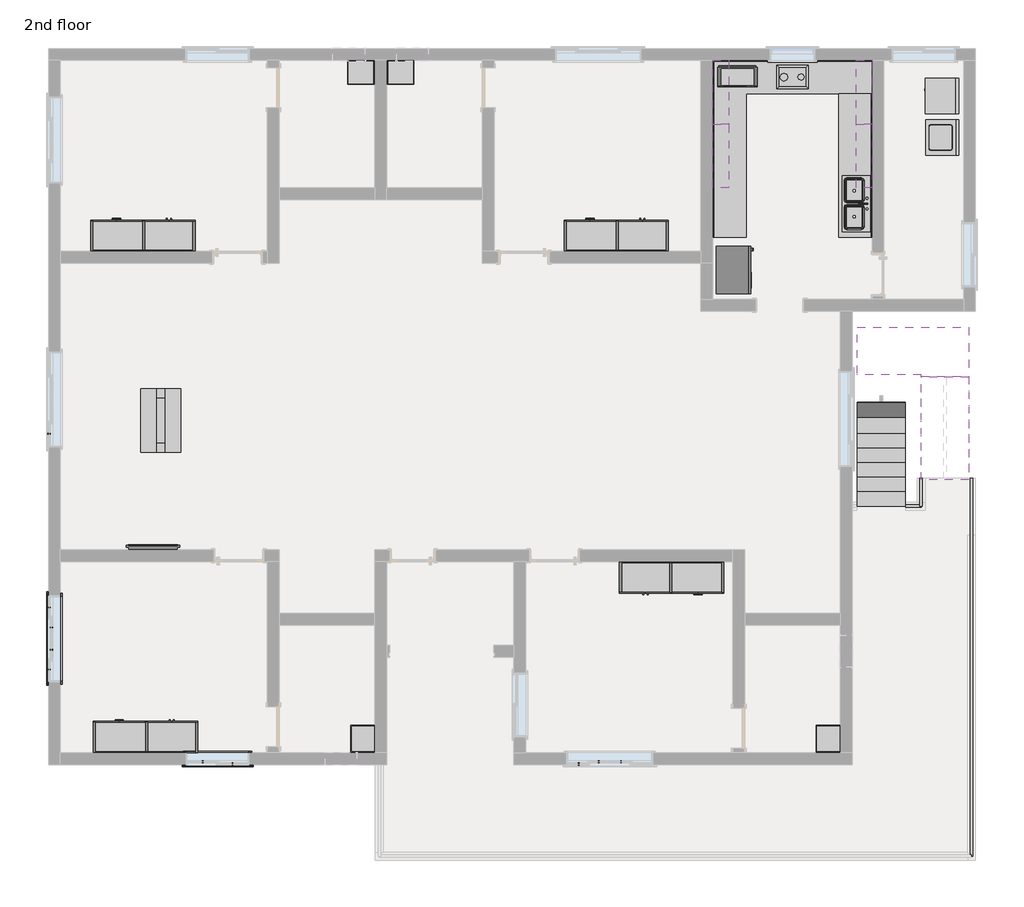
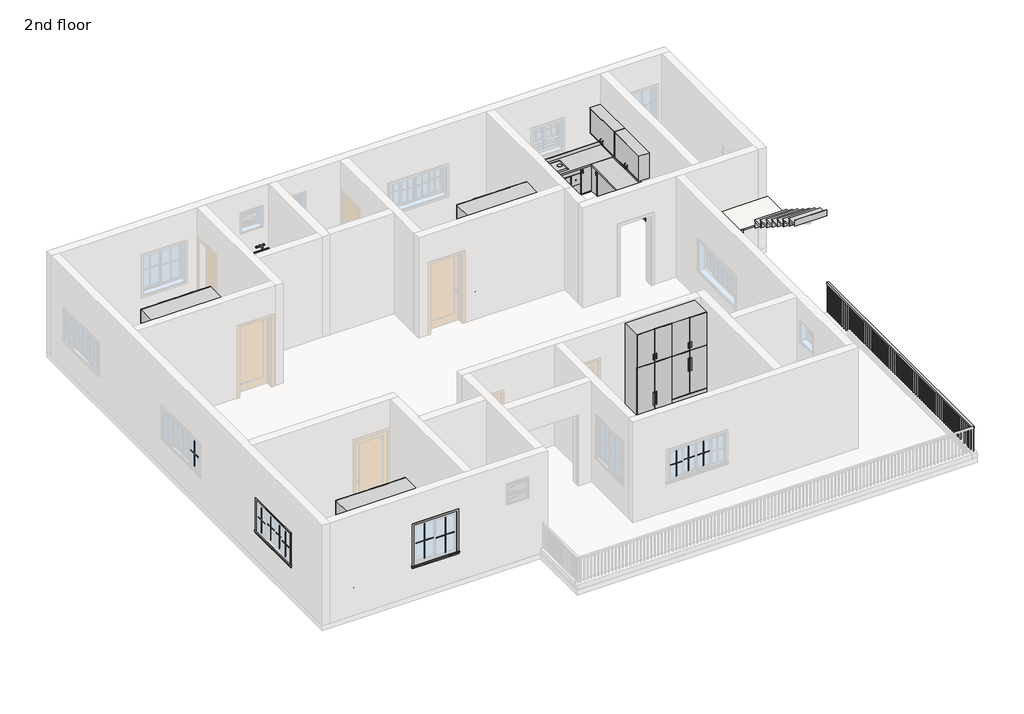
# One storey, part 3 of 4: 19 furniture elements, 18 proxies, 5 flow terminals, 3 railings, 2 stair flights, 1 slab.
# Revit data of these elements (continued)
# Elements 12, 13 (IfcBuildingElementProxy, "Muntin Pattern_2x2 : Muntin Pattern_2x2")
#   Width = 1' - 8 5/8"
#   Height = 3' - 6 1/4"
#   Interior Material = Wood - Stained
#   Exterior Material = Clad - White
#   Phase Created = New Construction
#   Materials on its faces: "Clad - White", "Wood - Stained"
# Element 14 (IfcBuildingElementProxy, "Trim-Window-Exterior-Flat : with Sill")
#   Opening Width = 5' - 5"
#   Opening Height = 3' - 0"
#   Trim Material = Clad - White
#   Phase Created = New Construction
#   Materials on its faces: "Clad - White"
# Element 15 (IfcBuildingElementProxy, "Trim-Window-Exterior-Flat : with Sill")
#   Opening Width = 4' - 0"
#   Opening Height = 4' - 0"
#   Trim Material = Clad - White
#   Phase Created = New Construction
#   Materials on its faces: "Clad - White"
# Element 16 (IfcBuildingElementProxy, "Trim-Window-Interior-Flat : Picture Frame")
#   Opening Width = 5' - 5"
#   Opening Height = 3' - 0"
#   Trim Material = Wood - Stained
#   Phase Created = New Construction
#   Materials on its faces: "Wood - Stained"
# Element 17 (IfcBuildingElementProxy, "Trim-Window-Interior-Flat : Picture Frame")
#   Opening Width = 4' - 0"
#   Opening Height = 4' - 0"
#   Trim Material = Wood - Stained
#   Phase Created = New Construction
#   Materials on its faces: "Wood - Stained"
# Element 18 (IfcBuildingElementProxy, "Washer : 27\" x 25\" x 35\"")
#   Phase Created = New Construction
#   Materials on its faces: "Metal - Paint Finish - Ivory,Matte"
# Element 19 (IfcFlowTerminal, "Sink - Work : 20\"x18\"")
#   Mark = "32"
#   Flow Pressure = 8.00 psi
#   Phase Created = New Construction
# Element 20 (IfcFlowTerminal, "Sink - Work : 20\"x18\"")
#   Mark = "33"
#   Flow Pressure = 8.00 psi
#   Phase Created = New Construction
# Element 21 (IfcFlowTerminal, "Sink - Work : 20\"x18\"")
#   Mark = "34"
#   Flow Pressure = 8.00 psi
#   Phase Created = New Construction
# Element 22 (IfcFlowTerminal, "Sink - Work : 20\"x18\"")
#   Mark = "35"
#   Flow Pressure = 8.00 psi
#   Phase Created = New Construction
# Element 23 (IfcFlowTerminal, "Sink Kitchen-Double : 42\" x 21\"")
#   Mark = "27"
#   Phase Created = New Construction
#   Materials on its faces: "Steel, Polished"
# Element 24 (IfcFurniture)
#   Phase Created = New Construction
#   Materials on its faces: "Default", "Default 3", "Default 2"
# Elements 25, 26, 27, 28 (IfcFurniture, "1Wardrobe_6271 : 1Wardrobe_6271")
#   Phase Created = New Construction
#   Materials on its faces: "Phase - Demo", "Default Wall", "Phase - Exist", "Default"
# Elements 29, 30, 31, 32 (IfcFurniture, "48\" 2")
#   Phase Created = New Construction
#   Materials on its faces: "Cabinets", "Cabinets - Handles"
# Elements 33, 34 (IfcFurniture, "Base Cabinet-Corner Unit-Square : 36\"")
#   Phase Created = New Construction
#   Materials on its faces: "Cabinets", "Cabinets - Handles"
# Element 35 (IfcFurniture, "Counter Top w Sink : 24\" Depth")
#   Sink Opening Width = 3' - 3"
#   Sink Opening Depth = 1' - 3"
#   Sink Location To Wall = 0' - 6"
#   Sink Location = 6' - 11"
#   Length = 9' - 0.36336"
#   Phase Created = New Construction
#   Materials on its faces: "Counter Top"
# Element 36 (IfcFurniture, "Counter Top-L Shaped : 24\" Depth")
#   Length - Leg 2 = 11' - 1.36336"
#   Length - Leg 1 = 10' - 0"
#   Phase Created = New Construction
#   Materials on its faces: "Counter Top"
# Element 37 (IfcFurniture, "Television-Plasma : 42\"")
#   Phase Created = New Construction
#   Materials on its faces: "Plastic - Gray", "Glass"
# Elements 38, 39, 40, 41 (IfcFurniture, "Upper Cabinet-Pass-Thru : 48\" x 30\" x 12\"")
#   Phase Created = New Construction
#   Materials on its faces: "Cabinet"
# Element 42 (IfcFurniture, "White_Modern_Coffee_Table_17067 : White_Modern_Coffee_Table_17067")
#   Phase Created = New Construction
#   Materials on its faces: "White Modern Coffee Table - Plastic", "White Modern Coffee Table - Wood"
# Elements 43, 44, 45 (IfcRailing, "Handrail - Rectangular")
#   Phase Created = New Construction
# Element 46 (IfcSlab, "Non-Monolithic Landing")
#   Phase Created = New Construction
# Elements 47, 48 (IfcStairFlight, "2\" Tread 1\" Nosing 1/4\" Riser")
#   Phase Created = New Construction
# Materials
#   "Metal - Chrome": colour RGB 17 17 17, transparency 0
#   "Metal - Steel, Polished": colour RGB 57 57 57, transparency 0
#   "Metal - Paint Finish - Ivory,Glossy": colour RGB 247 247 239, transparency 0
#   "Laminate - Ivory,Matte": colour RGB 247 247 239, transparency 0
#   "Metal - Paint Finish - Ivory,Matte": colour RGB 247 247 239, transparency 0
#   "Steel, Polished": class "Metal", colour RGB 192 192 192, transparency 0, Description = "Polished steel", Cost = 0
#   "Cabinets - Handles": class "Metal", colour RGB 57 57 57, transparency 0
#   "Cabinets": colour RGB 249 249 249, transparency 0
#   "Plastic - Gray": colour RGB 134 134 134, transparency 0
#   "White Modern Coffee Table - Wood": class "Generic", colour RGB 120 120 120, transparency 0, Cost = 0
#   "White Modern Coffee Table - Plastic": class "Generic", colour RGB 120 120 120, transparency 0, Cost = 0
#   "Glass": class "Glass", colour RGB 0 128 192, transparency 0.75, Description = "Soda Lime Glass", Cost = 0
#   "Clad - White": class "Wood", colour RGB 242 242 238, transparency 0, Cost = 0
#   "Wood - Stained": class "Wood", colour RGB 224 178 126, transparency 0, Cost = 0
#   "Default": colour RGB 127 127 127, transparency 0, Cost = 0
#   "Default 3": class "Glass", colour RGB 127 127 127, transparency 0
#   "Default 2": class "Plastic", colour RGB 127 127 127, transparency 0
#   "Phase - Demo": class "System", colour RGB 255 0 0, transparency 0.4, Cost = 0
#   "Default Wall": colour RGB 128 128 128, transparency 0, Cost = 0
#   "Phase - Exist": class "System", colour RGB 127 127 127, transparency 0, Cost = 0
#   "Counter Top": class "Wood", colour RGB 226 177 128, transparency 0
#   "Cabinet": colour RGB 204 122 2, transparency 0
